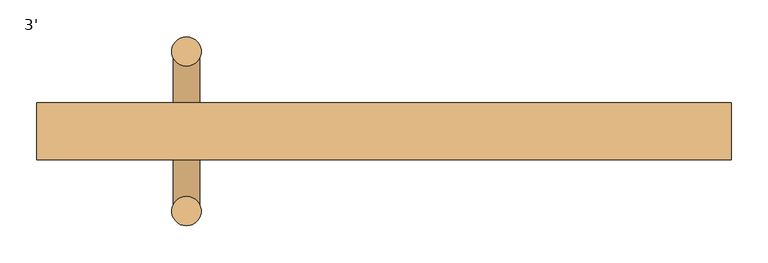
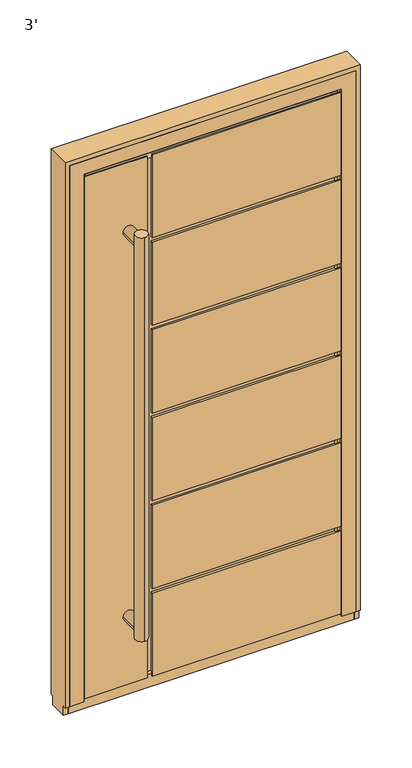
"""IFC4 building model written with IfcOpenShell, lengths in millimetres: door geometry, 3'."""

from ifc_helpers import new_model, si_unit, point, frame, frame_2d, origin, place, context, project, spatial, circle_curve, trimmed, segment, composite_curve, outline, extrude, faceted_brep, source, transform, mapped, element, save


def door_3_3562bf2b(model_context):
    return source(origin(), model_context, "Body", "SolidModel", [
        extrude(outline(composite_curve([segment(trimmed(circle_curve(frame_2d((-268.65, 52.7003001)), 20.0), [point((-268.65, 32.7003001))], [point((-268.65, 72.7003001))], False, "CARTESIAN"), True, "CONTINUOUS"), segment(trimmed(circle_curve(frame_2d((-268.65, 52.7003001)), 20.0), [point((-268.65, 72.7003001))], [point((-268.65, 32.7003001))], False, "CARTESIAN"), True, "CONTINUOUS")], self_intersect=False)), frame((0.0, 0.0, 210.0000003), z_axis=(0.0, 0.0, 1.0), x_axis=(1.0, 0.0, 0.0)), (0.0, 0.0, 1.0), 1363.8),
        extrude(outline(composite_curve([segment(trimmed(circle_curve(frame_2d((-268.65, -164.3003001)), 20.0), [point((-268.65, -184.3003001))], [point((-268.65, -144.3003001))], False, "CARTESIAN"), True, "CONTINUOUS"), segment(trimmed(circle_curve(frame_2d((-268.65, -164.3003001)), 20.0), [point((-268.65, -144.3003001))], [point((-268.65, -184.3003001))], False, "CARTESIAN"), True, "CONTINUOUS")], self_intersect=False)), frame((0.0, 0.0, 210.0000003), z_axis=(0.0, 0.0, 1.0), x_axis=(1.0, 0.0, 0.0)), (0.0, 0.0, 1.0), 1363.8),
        extrude(outline(composite_curve([segment(trimmed(circle_curve(frame_2d((241.9000003, -268.65)), 18.0), [point((241.9000003, -286.65))], [point((241.9000003, -250.65))], False, "CARTESIAN"), True, "CONTINUOUS"), segment(trimmed(circle_curve(frame_2d((241.9000003, -268.65)), 18.0), [point((241.9000003, -250.65))], [point((241.9000003, -286.65))], False, "CARTESIAN"), True, "CONTINUOUS")], self_intersect=False)), frame((0.0, -164.3, 0.0), z_axis=(0.0, 1.0, 0.0), x_axis=(0.0, 0.0, 1.0)), (0.0, 0.0, 1.0), 217.0),
        extrude(outline(composite_curve([segment(trimmed(circle_curve(frame_2d((1541.9000003, -268.65)), 18.0), [point((1541.9000003, -286.65))], [point((1541.9000003, -250.65))], False, "CARTESIAN"), True, "CONTINUOUS"), segment(trimmed(circle_curve(frame_2d((1541.9000003, -268.65)), 18.0), [point((1541.9000003, -250.65))], [point((1541.9000003, -286.65))], False, "CARTESIAN"), True, "CONTINUOUS")], self_intersect=False)), frame((0.0, -164.3, 0.0), z_axis=(0.0, 1.0, 0.0), x_axis=(0.0, 0.0, 1.0)), (0.0, 0.0, 1.0), 217.0),
        faceted_brep([(-193.65, -24.3, 306.466667), (383.65, -24.3, 306.466667), (383.65, -24.3, 291.466667), (-193.65, -24.3, 291.466667), (-193.65, -24.3, 35.0), (-208.65, -24.3, 35.0), (-208.65, -24.3, 1748.8000003), (-193.65, -24.3, 1748.8000003), (-193.65, -24.3, 1492.3333337), (383.65, -24.3, 1492.3333337), (383.65, -24.3, 1477.3333337), (-193.65, -24.3, 1477.3333337), (-193.65, -24.3, 1195.866667), (383.65, -24.3, 1195.866667), (383.65, -24.3, 1180.866667), (-193.65, -24.3, 1180.866667), (-193.65, -24.3, 899.4000004), (383.65, -24.3, 899.4000004), (383.65, -24.3, 884.4000004), (-193.65, -24.3, 884.4000004), (-193.65, -24.3, 602.9333337), (383.65, -24.3, 602.9333337), (383.65, -24.3, 587.9333337), (-193.65, -24.3, 587.9333337), (-193.65, -17.3, 587.9333337), (-193.65, -17.3, 306.466667), (383.65, -17.3, 587.9333337), (383.65, -26.3002302, 1748.8000003), (383.65, -26.3002302, 35.0), (383.65, -19.2979528, 35.0), (383.65, -19.2979528, 24.0), (383.65, -17.3, 24.0), (383.65, -17.3, 291.466667), (383.65, -17.3, 306.466667), (383.65, -17.3, 602.9333337), (383.65, -17.3, 884.4000004), (383.65, -17.3, 899.4000004), (383.65, -17.3, 1180.866667), (383.65, -17.3, 1195.866667), (383.65, -17.3, 1477.3333337), (383.65, -17.3, 1492.3333337), (383.65, -17.3, 1748.8000003), (-193.65, -17.3, 602.9333337), (-193.65, -17.3, 884.4000004), (-193.65, -17.3, 899.4000004), (-193.65, -17.3, 1180.866667), (-208.65, -19.2979528, 35.0), (-208.65, -19.2979528, 24.0), (-208.65, -17.3, 24.0), (-208.65, -17.3, 1748.8000003), (-383.65, -26.3002302, 35.0), (-383.65, -19.2979528, 35.0), (-193.65, -19.2979528, 35.0), (-193.65, -17.3, 291.466667), (-193.65, -17.3, 24.0), (-193.65, -19.2979528, 24.0), (-383.65, -19.2979528, 24.0), (-383.65, -17.3, 24.0), (-383.65, -17.3, 1748.8000003), (-193.65, -17.3, 1195.866667), (-193.65, -17.3, 1477.3333337), (-193.65, -17.3, 1492.3333337), (-193.65, -17.3, 1748.8000003), (408.65, -94.3, 10.0000003), (-193.65, -94.3, 10.0000003), (-193.65, -91.3, 10.0000003), (408.65, -91.3, 10.0000003), (-408.65, -91.3, 10.0000003), (-208.65, -91.3, 10.0000003), (-208.65, -94.3, 10.0000003), (-408.65, -94.3, 10.0000003), (408.65, -94.3, 306.466667), (408.65, -91.3, 306.466667), (408.65, -91.3, 587.9333337), (408.65, -94.3, 587.9333337), (408.65, -94.3, 899.4000004), (408.65, -91.3, 899.4000004), (408.65, -91.3, 1180.866667), (408.65, -94.3, 1180.866667), (408.65, -94.3, 602.9333337), (408.65, -91.3, 602.9333337), (408.65, -91.3, 884.4000004), (408.65, -94.3, 884.4000004), (408.65, -94.3, 1195.866667), (408.65, -91.3, 1195.866667), (408.65, -91.3, 1477.3333337), (408.65, -94.3, 1477.3333337), (408.65, -94.3, 1773.8000003), (408.65, -94.3, 1492.3333337), (408.65, -91.3, 1492.3333337), (408.65, -91.3, 1773.8000003), (408.65, -91.3, 291.466667), (408.65, -94.3, 291.466667), (-193.65, -91.3, 25.5), (393.15, -91.3, 25.5), (393.15, -91.3, 291.466667), (393.15, -91.3, 306.466667), (393.15, -91.3, 587.9333337), (393.15, -91.3, 899.4000004), (393.15, -91.3, 1180.866667), (393.15, -91.3, 602.9333337), (393.15, -91.3, 884.4000004), (-393.15, -91.3, 25.5), (-208.65, -91.3, 25.5), (-408.65, -91.3, 1773.8000003), (-208.65, -91.3, 1773.8000003), (-208.65, -91.3, 1758.3000003), (-393.15, -91.3, 1758.3000003), (393.15, -91.3, 1195.866667), (393.15, -91.3, 1477.3333337), (393.15, -91.3, 1492.3333337), (393.15, -91.3, 1758.3000003), (-193.65, -91.3, 1758.3000003), (-193.65, -91.3, 1773.8000003), (-193.65, -87.3, 291.466667), (-193.65, -87.3, 25.5), (-193.65, -94.3, 291.466667), (-208.65, -94.3, 1773.8000003), (-408.65, -94.3, 1773.8000003), (-193.65, -94.3, 587.9333337), (-193.65, -94.3, 306.466667), (-193.65, -94.3, 1180.866667), (-193.65, -94.3, 899.4000004), (-193.65, -94.3, 884.4000004), (-193.65, -94.3, 602.9333337), (-193.65, -94.3, 1477.3333337), (-193.65, -94.3, 1195.866667), (-193.65, -94.3, 1773.8000003), (-193.65, -94.3, 1492.3333337), (-208.65, -87.3, 1758.3000003), (-208.65, -87.3, 25.5), (-383.65, -26.3002302, 1748.8000003), (393.15, -26.3002302, 1758.3000003), (393.15, -26.3002302, 25.5), (-393.15, -26.3002302, 25.5), (-393.15, -26.3002302, 1758.3000003), (393.15, -87.3, 1492.3333337), (393.15, -87.3, 1477.3333337), (393.15, -87.3, 1195.866667), (393.15, -87.3, 1180.866667), (393.15, -87.3, 899.4000004), (393.15, -87.3, 884.4000004), (393.15, -87.3, 602.9333337), (393.15, -87.3, 587.9333337), (393.15, -87.3, 306.466667), (393.15, -87.3, 291.466667), (-193.65, -87.3, 1477.3333337), (-193.65, -87.3, 1492.3333337), (-193.65, -87.3, 1758.3000003), (-193.65, -87.3, 306.466667), (-193.65, -87.3, 587.9333337), (-193.65, -87.3, 602.9333337), (-193.65, -87.3, 884.4000004), (-193.65, -87.3, 899.4000004), (-193.65, -87.3, 1180.866667), (-193.65, -87.3, 1195.866667)], [[[0, 1, 2, 3, 4, 5, 6, 7, 8, 9, 10, 11, 12, 13, 14, 15, 16, 17, 18, 19, 20, 21, 22, 23]], [[23, 24, 25, 0]], [[23, 22, 26, 24]], [[27, 28, 29, 30, 31, 32, 2, 1, 33, 26, 22, 21, 34, 35, 18, 17, 36, 37, 14, 13, 38, 39, 10, 9, 40, 41]], [[42, 34, 21, 20]], [[19, 43, 42, 20]], [[19, 18, 35, 43]], [[44, 36, 17, 16]], [[15, 45, 44, 16]], [[5, 46, 47, 48, 49, 6]], [[28, 50, 51, 46, 5, 4, 52, 29]], [[53, 54, 55, 52, 4, 3]], [[3, 2, 32, 53]], [[25, 33, 1, 0]], [[29, 52, 55, 30]], [[56, 47, 46, 51]], [[30, 55, 54, 31]], [[57, 48, 47, 56]], [[36, 44, 45, 37]], [[34, 42, 43, 35]], [[33, 25, 24, 26]], [[54, 53, 32, 31]], [[58, 49, 48, 57]], [[38, 59, 60, 39]], [[41, 40, 61, 62]], [[63, 64, 65, 66]], [[67, 68, 69, 70]], [[71, 72, 73, 74]], [[75, 76, 77, 78]], [[79, 80, 81, 82]], [[83, 84, 85, 86]], [[87, 88, 89, 90]], [[66, 91, 92, 63]], [[65, 93, 94, 95, 91, 66]], [[72, 96, 97, 73]], [[76, 98, 99, 77]], [[80, 100, 101, 81]], [[102, 103, 68, 67, 104, 105, 106, 107]], [[84, 108, 109, 85]], [[90, 89, 110, 111, 112, 113]], [[114, 115, 93, 65, 64, 116]], [[70, 69, 117, 118]], [[63, 92, 116, 64]], [[74, 119, 120, 71]], [[78, 121, 122, 75]], [[82, 123, 124, 79]], [[86, 125, 126, 83]], [[87, 127, 128, 88]], [[70, 118, 104, 67]], [[129, 106, 105, 117, 69, 68, 103, 130]], [[58, 57, 56, 51, 50, 131]], [[132, 133, 134, 135], [131, 50, 28, 27]], [[111, 110, 136, 137, 109, 108, 138, 139, 99, 98, 140, 141, 101, 100, 142, 143, 97, 96, 144, 145, 95, 94, 133, 132]], [[94, 93, 115, 130, 103, 102, 134, 133]], [[135, 134, 102, 107]], [[146, 137, 136, 147, 148, 129, 130, 115, 114, 145, 144, 149, 150, 143, 142, 151, 152, 141, 140, 153, 154, 139, 138, 155]], [[153, 122, 121, 154]], [[153, 140, 98, 76, 75, 122]], [[123, 82, 81, 101, 141, 152]], [[151, 124, 123, 152]], [[151, 142, 100, 80, 79, 124]], [[119, 74, 73, 97, 143, 150]], [[149, 120, 119, 150]], [[149, 144, 96, 72, 71, 120]], [[116, 92, 91, 95, 145, 114]], [[15, 14, 37, 45]], [[59, 38, 13, 12]], [[11, 60, 59, 12]], [[11, 10, 39, 60]], [[61, 40, 9, 8]], [[8, 7, 62, 61]], [[125, 86, 85, 109, 137, 146]], [[128, 127, 113, 112, 148, 147]], [[121, 78, 77, 99, 139, 154]], [[155, 138, 108, 84, 83, 126]], [[155, 126, 125, 146]], [[147, 136, 110, 89, 88, 128]], [[90, 113, 127, 87]], [[118, 117, 105, 104]], [[132, 135, 107, 106, 129, 148, 112, 111]], [[27, 41, 62, 7, 6, 49, 58, 131]]]),
        faceted_brep([(-457.2, -94.3, 0.0), (-457.2, -85.2997571, 0.0), (-412.7, -85.2997571, 0.0), (-412.7, -94.3, 0.0), (-403.2, -21.8000042, 0.0), (-403.2, -26.3, 0.0), (-457.2, -26.3, 0.0), (-457.2, -17.3, 0.0), (-387.7, -17.3, 0.0), (-387.7, -21.8000042, 0.0), (457.2, -17.3, 0.0), (457.2, -26.3, 0.0), (403.2, -26.3, 0.0), (403.2, -21.8000042, 0.0), (387.7, -21.8000042, 0.0), (387.7, -17.3, 0.0), (412.7, -85.2997571, 0.0), (457.2, -85.2997571, 0.0), (457.2, -94.3, 0.0), (412.7, -94.3, 0.0), (-457.2, -26.3, -30.0), (-457.2, -85.2997571, -30.0), (-457.2, -94.3, 1828.8), (-457.2, -17.3, 1828.8), (-412.7, -94.3, 1784.3), (412.7, -94.3, 1784.3), (457.2, -94.3, 1828.8), (457.2, -17.3, 1828.8), (457.2, -85.2997571, -30.0), (457.2, -26.3, -30.0), (387.7, -17.3, 1759.3), (-387.7, -17.3, 1759.3), (-403.2, -85.3, 1774.8), (-403.2, -85.3, 14.5), (-403.2, -26.3, 14.5), (-403.2, -21.8000042, 1774.8), (403.2, -21.8000042, 1774.8), (403.2, -85.3, 1774.8), (403.2, -26.3, 14.5), (403.2, -85.3, 14.5), (-412.7, -85.3, 1784.3), (412.7, -85.3, 1784.3), (-387.7, -21.8000042, 1759.3), (387.7, -21.8000042, 1759.3)], [[[0, 1, 2, 3]], [[4, 5, 6, 7, 8, 9]], [[10, 11, 12, 13, 14, 15]], [[16, 17, 18, 19]], [[7, 6, 20, 21, 1, 0, 22, 23]], [[3, 24, 25, 19, 18, 26, 22, 0]], [[22, 26, 27, 23]], [[18, 17, 28, 29, 11, 10, 27, 26]], [[7, 23, 27, 10, 15, 30, 31, 8]], [[32, 33, 34, 5, 4, 35]], [[35, 36, 37, 32]], [[36, 13, 12, 38, 39, 37]], [[40, 24, 3, 2]], [[16, 41, 40, 2, 1, 21, 28, 17], [37, 39, 33, 32]], [[9, 42, 43, 14, 13, 36, 35, 4]], [[8, 31, 42, 9]], [[24, 40, 41, 25]], [[30, 43, 42, 31]], [[19, 25, 41, 16]], [[14, 43, 30, 15]], [[20, 6, 5, 34, 38, 12, 11, 29]], [[39, 38, 34, 33]], [[20, 29, 28, 21]]]),
        faceted_brep([(-457.2, -85.3, -30.0), (-472.2, -85.3, -30.0), (-472.2, -26.3, -30.0), (-457.2, -26.3, -30.0), (-457.2, -94.3, 1828.8), (-457.2, -94.3, 0.0), (-457.2, -85.3, 0.0), (-457.2, -26.3, 0.0), (-457.2, -17.3, 0.0), (-457.2, -17.3, 1828.8), (-472.2, -26.3, 0.0), (472.2, -26.3, 0.0), (472.2, -26.3, -30.0), (457.2, -26.3, -30.0), (457.2, -26.3, 0.0), (-472.2, -17.3, 1843.8), (-472.2, -17.3, 0.0), (-472.2, -85.3, 0.0), (-472.2, -94.3, 0.0), (-472.2, -94.3, 1843.8), (457.2, -85.3, 0.0), (457.2, -85.3, -30.0), (472.2, -85.3, -30.0), (472.2, -85.3, 0.0), (457.2, -17.3, 1828.8), (457.2, -17.3, 0.0), (457.2, -94.3, 0.0), (457.2, -94.3, 1828.8), (472.2, -94.3, 0.0), (472.2, -94.3, 1843.8), (472.2, -17.3, 0.0), (472.2, -17.3, 1843.8)], [[[0, 1, 2, 3]], [[4, 5, 6, 0, 3, 7, 8, 9]], [[7, 3, 2, 10]], [[11, 12, 13, 14]], [[15, 16, 10, 2, 1, 17, 18, 19]], [[17, 1, 0, 6]], [[20, 21, 22, 23]], [[24, 25, 14, 13, 21, 20, 26, 27]], [[27, 26, 28, 29, 19, 18, 5, 4]], [[6, 5, 18, 17]], [[23, 28, 26, 20]], [[22, 21, 13, 12]], [[10, 16, 8, 7]], [[14, 25, 30, 11]], [[9, 8, 16, 15, 31, 30, 25, 24]], [[29, 28, 23, 22, 12, 11, 30, 31]], [[9, 24, 27, 4]], [[19, 29, 31, 15]]]),
    ])


if __name__ == "__main__":
    model = new_model("IFC4")
    model_context = context("Model", 3, world=origin())
    ifc_project = project(units=[si_unit("LENGTHUNIT", "METRE", prefix="MILLI")], contexts=[model_context])
    site = spatial("IfcSite", under=ifc_project)
    building = spatial("IfcBuilding", under=site)
    placement = place(None, origin())
    door_3_shape = door_3_3562bf2b(model_context)
    element("IfcDoor", 1, ObjectType="3'", at=placement, inside=building, context=model_context, shape_type="MappedRepresentation", body=[
        mapped(door_3_shape, transform((0.0, 0.0, 0.0), x_axis=(1.0, 0.0, 0.0), y_axis=(0.0, 1.0, 0.0), z_axis=(0.0, 0.0, 1.0))),
    ])
    save(model, "model.ifc")

# Revit data of these elements
# Type "3'"
#   Type Mark = "41"
#   Water resistance = "up to Class E900, EN 12208:2001"
#   Uniclass2015Version = "v1.21"
#   Uniclass2015Reference = "Ss_25_30_20_30"
#   Uniclass2015Description = "Frame and door leaf system"
#   URL = "www.aluprof.com"
#   Type IFC Predefined Type = "USERDEFINED"
#   Right-hand / Left-hand door [instance default] = ""
#   Resistance to wind load = "up to Class C5/B5, EN 12210:2001"
#   Insert type = "ST"
#   Hardware [instance default] = ""
#   Product page = "https://aluprof.com/en/architects/offer/window-and-door-systems/panel-doors#visualisation"
#   Operation = "SinglePanelOutwardOpening"
#   Opening type = "Outward"
#   NBSReference = "25-50-20/125"
#   NBSDescription = "Frame and door leaf system"
#   Important = "The actual acceptable construction dimensions are dependent on the selection of profiles and hardware, glazing type, construction weight and the construction’s operating conditions. These should be determined by a suitably qualified person, and using ALUPROF’s calculation software"
#   IfcExportType = "USERDEFINED"
#   IfcExportAs = "IfcDoorType"
#   Handle type [instance default] = ""
#   Manufacturer = "ALUPROF SA"
#   Export Type to IFC As = "IfcDoorType"
#   Door sill type [instance default] = ""
#   Description = "External single-leaf panel door outward opening"
#   Model = "MB-86 ST Panel Door AD07"
#   Content of the recyclate in the material = "69.2%"
#   COBie.Type.WarrantyDurationParts = ""
#   COBie.Type.Name = ""
#   COBie.Type.Manufacturer = "ALUPROF SA"
#   COBie.Space.Name = ""
#   COBie.Floor.Name = ""
#   COBie.Facility.Name = ""
#   COBie.CreatedOn = ""
#   COBie.Component.WarrantyStartDate = ""
#   COBie.Component.Name = "MB-86 ST Panel Door AD07"
#   Burglar resistance = "RC2"
#   Air permeability = "up to Class 4, EN 12207:2001"
#   Width of the active leaf = 2' - 8.17717"
#   Placement in wall = 0' - 0.7874"
#   Thickness = 0' - 3.0315"
#   Height of the opening sash = 5' - 9.44094"
#   Handle Offset = 3' - 5.33858"
#   Rough Height = 6' - 2.40945"
#   Rough Width = 3' - 1.1811"
#   Height = 6' - 0"
#   Width = 3' - 0"
#   Construction depth = 0' - 3.0315"
#   Clear opening width = 2' - 3.94882"
#   Clear opening height = 5' - 8.47638"
#   Height of the array = 0' - 11.08136"
#   Schedule No. [instance default] = 1
#   Handrail [instance default] = yes
#   IsExternal = yes
#   Handle [instance default] = no
#   Door closer [instance default] = no
#   Function = 1
#   COBie.Type = yes
#   COBie = yes
#   Access control [instance default] = no
#   Panel = element 371215
#   Wall Closure = (empty or 0)
